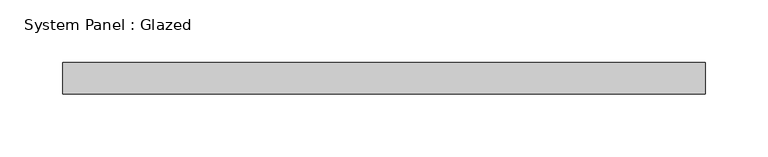
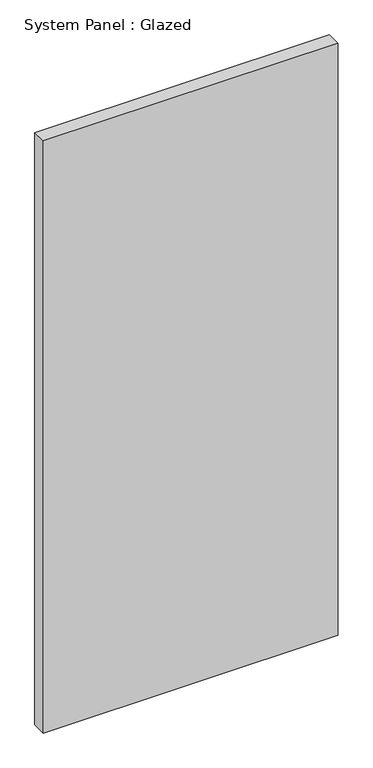
"""IFC4 building model written with IfcOpenShell, lengths in millimetres: plate geometry, System Panel : Glazed."""

from ifc_helpers import new_model, si_unit, origin, origin_with_axes, place, context, project, spatial, polyline, outline, extrude, source, transform, mapped, element, save


def system_panel_glazed_1715a493(model_context):
    return source(origin(), model_context, "Body", "SweptSolid", [
        extrude(outline(polyline([(257.175, 19.05), (-257.175, 19.05), (-257.175, 44.45), (257.175, 44.45), (257.175, 19.05)])), origin_with_axes(), (0.0, 0.0, 1.0), 1092.2),
    ])


if __name__ == "__main__":
    model = new_model("IFC4")
    model_context = context("Model", 3, world=origin())
    ifc_project = project(units=[si_unit("LENGTHUNIT", "METRE", prefix="MILLI")], contexts=[model_context])
    site = spatial("IfcSite", under=ifc_project)
    building = spatial("IfcBuilding", under=site)
    placement = place(None, origin())
    system_panel_glazed_shape = system_panel_glazed_1715a493(model_context)
    element("IfcPlate", 1, ObjectType="System Panel : Glazed", at=placement, inside=building, context=model_context, shape_type="MappedRepresentation", body=[
        mapped(system_panel_glazed_shape, transform((0.0, 0.0, 0.0), x_axis=(1.0, 0.0, 0.0), y_axis=(0.0, 1.0, 0.0), z_axis=(0.0, 0.0, 1.0))),
    ])
    save(model, "model.ifc")

# Revit data of these elements
# Type "System Panel : Glazed"
#   Construction Type Id = "GSP4R"
#   Analytic Construction = "1/8 in Pilkington single glazing"
#   Visual Light Transmittance = 0.9
#   Solar Heat Gain Coefficient = 0.86
#   Heat Transfer Coefficient (U) = 1.18115 BTU/(h·ft²·°F)
#   Define Thermal Properties by = 1
# Element 1 (IfcPlate, "System Panel : Glazed")
#   Materials on its faces: "Glass"
# Materials
#   "Glass": class "Glass", colour RGB 0 128 192, transparency 0.75, Description = "Soda Lime Glass", Cost = 0
